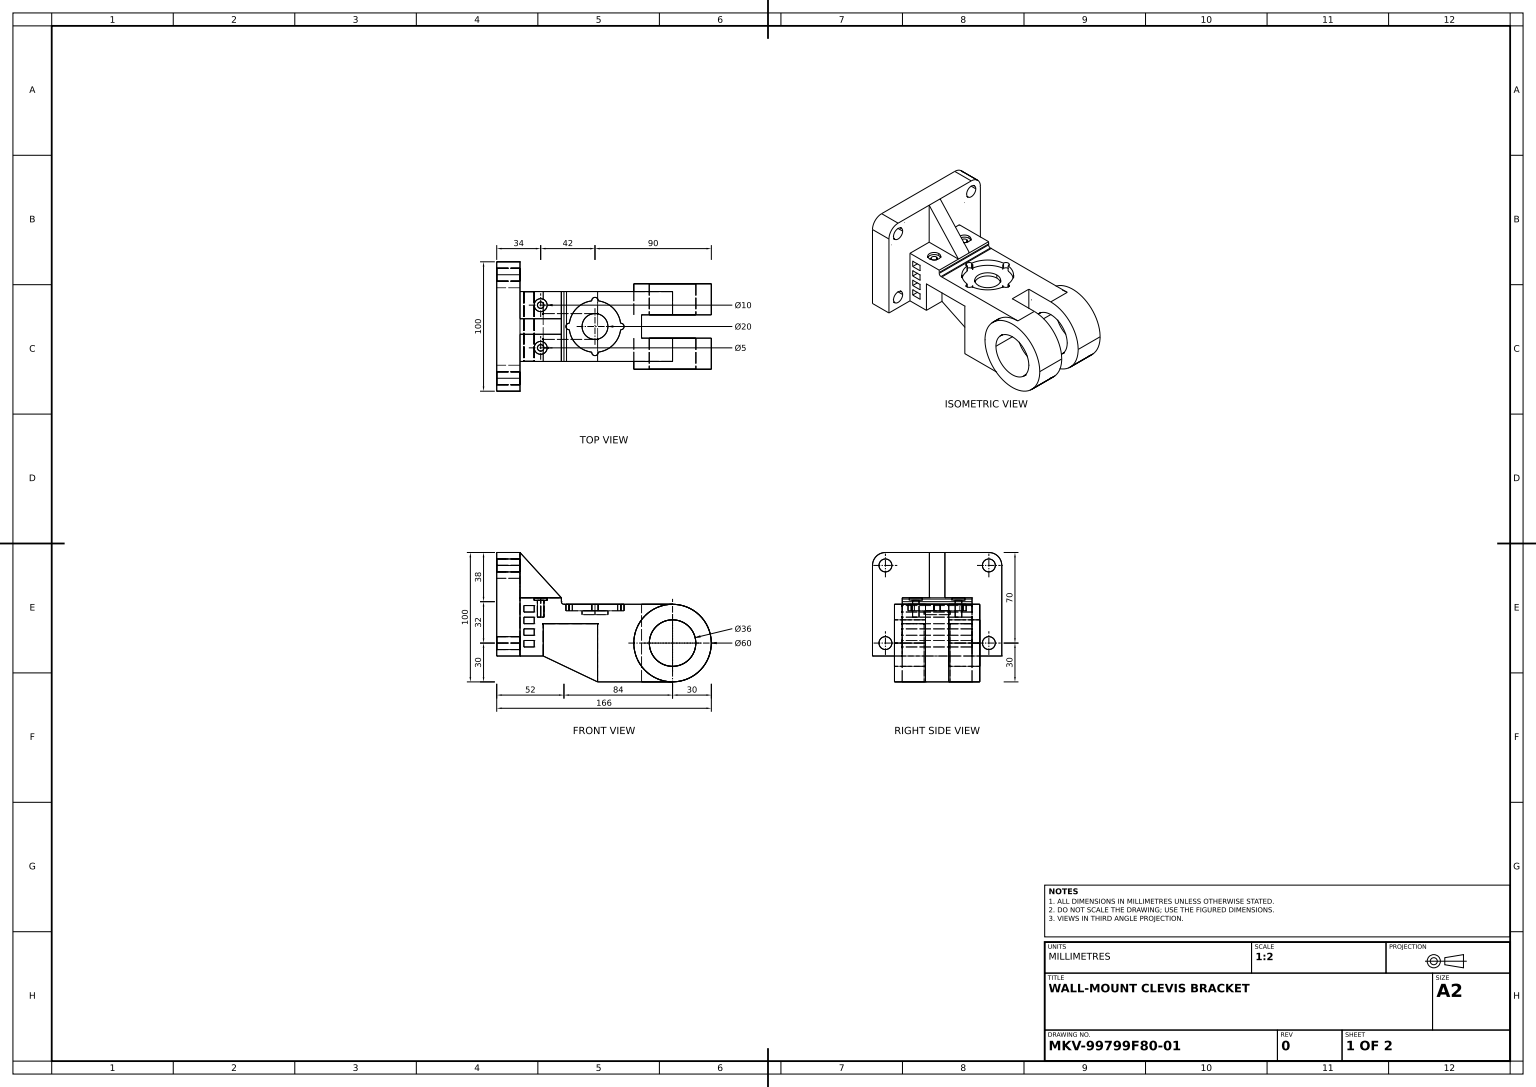
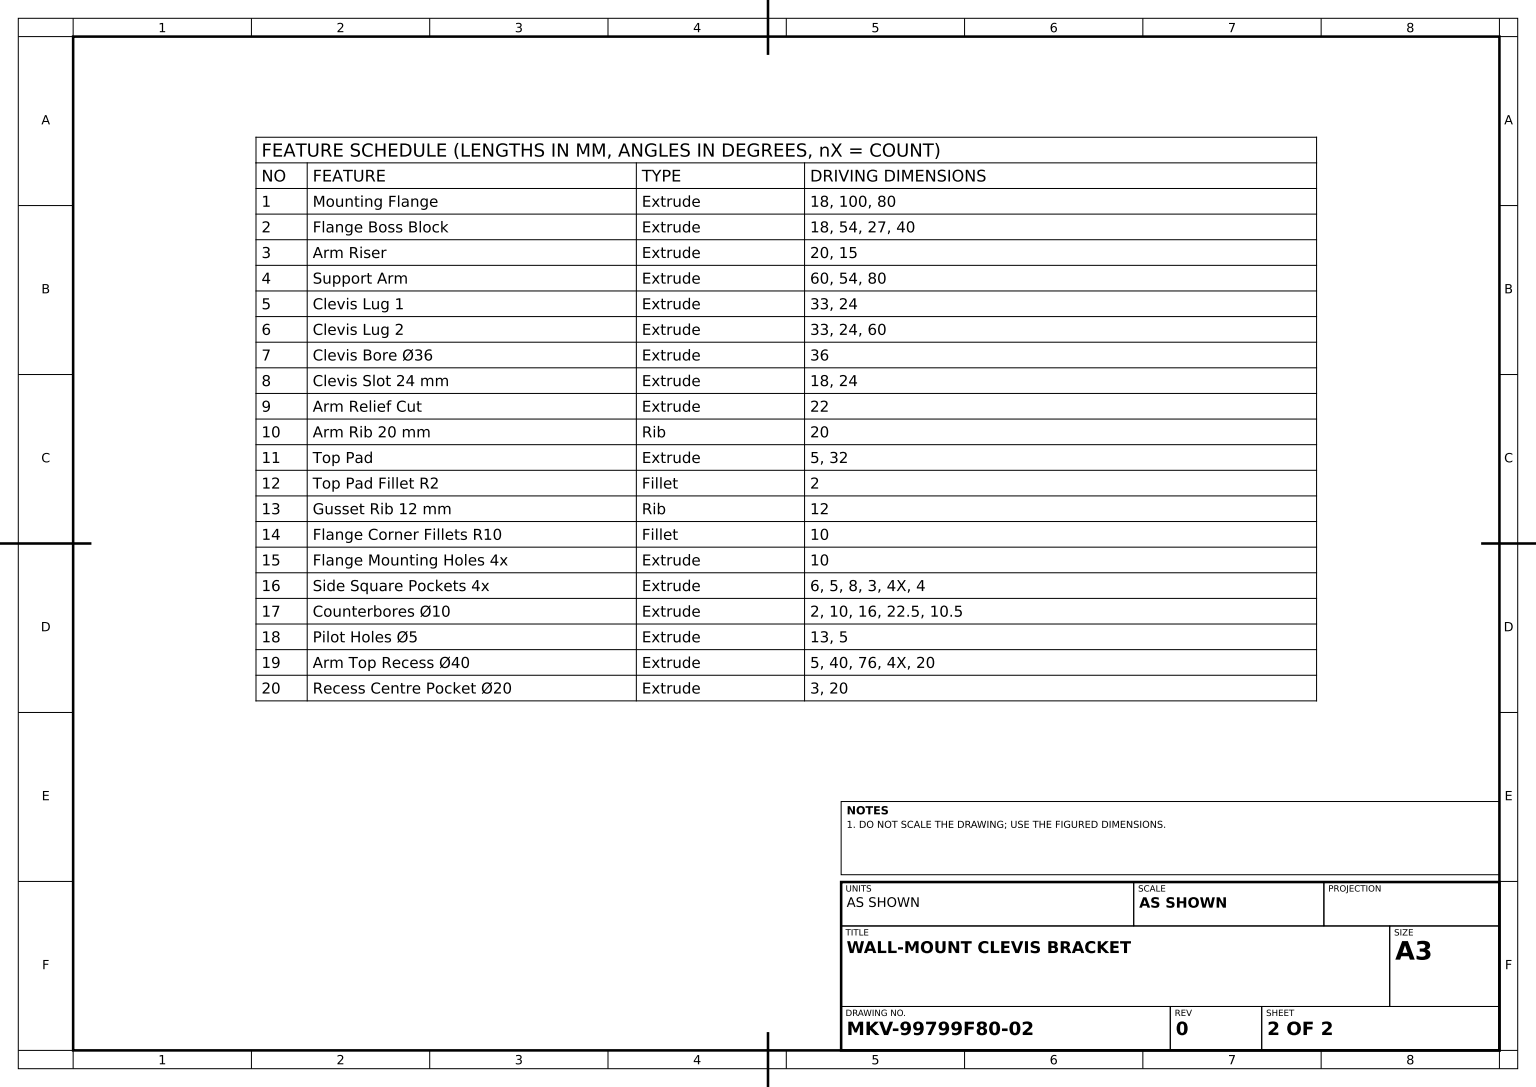
from build123d import *

# Parameters (mm, degrees)
MOUNTING_FLANGE_SKETCH_W          = 100
MOUNTING_FLANGE_SKETCH_H          = 80
MOUNTING_FLANGE_DEPTH             = 18
FLANGE_BOSS_BLOCK_SKETCH_W        = 54
FLANGE_BOSS_BLOCK_SKETCH_H        = 40
FLANGE_BOSS_BLOCK_DEPTH           = 18
ARM_RISER_SKETCH_W                = 54
ARM_RISER_SKETCH_H                = 15
ARM_RISER_DEPTH                   = 20
SUPPORT_ARM_SKETCH_W              = 80
SUPPORT_ARM_SKETCH_H              = 54
SUPPORT_ARM_DEPTH                 = 60
CLEVIS_LUG_1_SKETCH_R             = 30
CLEVIS_LUG_1_DEPTH                = 24
CLEVIS_START                      = 24
CLEVIS_LUG_2_SKETCH_R             = 30
CLEVIS_LUG_2_DEPTH                = 24
CLEVIS_BORE_SKETCH_R              = 18
CLEVIS_BORE_36_DEPTH              = 196.05127531
CLEVIS_SLOT_SKETCH_W              = 24
CLEVIS_SLOT_SKETCH_H              = 18
CLEVIS_SLOT_24_MM_DEPTH           = 184.455716727
ARM_RELIEF_CUT_SKETCH_W           = 22
ARM_RELIEF_CUT_SKETCH_H           = 45
ARM_RELIEF_CUT_DEPTH              = 193.574660846
ARM_RIB_20_MM_REACH               = 185.456
ARM_RIB_SKETCH_WALL_W             = 415.430246854
ARM_RIB_SKETCH_WALL_H             = 20
TOP_PAD_SKETCH_W                  = 32
TOP_PAD_SKETCH_H                  = 54
TOP_PAD_DEPTH                     = 5
TOP_PAD_FILLET_R2_R               = 2
GUSSET_RIB_12_MM_REACH            = 185.456
GUSSET_RIB_SKETCH_WALL_W          = 416.33505626
GUSSET_RIB_SKETCH_WALL_H          = 12
FLANGE_CORNER_FILLETS_R10_R       = 10
FLANGE_MOUNTING_HOLES_SKETCH_R    = 5
FLANGE_MOUNTING_HOLES_4X_DEPTH    = 168.343957166
SIDE_SQUARE_POCKETS_4X_DEPTH      = 193.574660846
SIDE_SQUARE_POCKETS_4X_DEPTH_BACK = 193.574660846
SIDE_SQUARE_POCKETS_SKETCH_W      = 8
SIDE_SQUARE_POCKETS_SKETCH_H      = 5
COUNTERBORE_SKETCH_R              = 5
COUNTERBORES_10_DEPTH             = 2
PILOT_HOLES_SKETCH_R              = 2.5
PILOT_HOLES_5_DEPTH               = 13
ARM_TOP_RECESS_40_DEPTH           = 5
RECESS_CENTRE_POCKET_SKETCH_R     = 10
RECESS_CENTRE_POCKET_20_DEPTH     = 3


with BuildPart() as part:
    # Mounting Flange Sketch → Mounting Flange (new body)
    with BuildSketch(Plane(origin=(0, 0, 0), x_dir=(0, 0, -1), z_dir=(1, 0, 0))):
        Rectangle(MOUNTING_FLANGE_SKETCH_W, MOUNTING_FLANGE_SKETCH_H)
    extrude(amount=MOUNTING_FLANGE_DEPTH)

    # Flange Boss Block Sketch → Flange Boss Block (add)
    with BuildSketch(Plane(origin=(18, 0, 0), x_dir=(0, 0, -1), z_dir=(1, 0, 0))):
        with Locations((0, -20)):
            Rectangle(FLANGE_BOSS_BLOCK_SKETCH_W, FLANGE_BOSS_BLOCK_SKETCH_H)
    extrude(amount=FLANGE_BOSS_BLOCK_DEPTH)

    # Arm Riser Sketch → Arm Riser (add)
    with BuildSketch(Plane(origin=(36, 0, 0), x_dir=(0, 0, -1), z_dir=(1, 0, 0))):
        with Locations((0, -7.5)):
            Rectangle(ARM_RISER_SKETCH_W, ARM_RISER_SKETCH_H)
    extrude(amount=ARM_RISER_DEPTH)

    # Support Arm Sketch → Support Arm (add)
    with BuildSketch(Plane(origin=(0, 0, 0), x_dir=(1, 0, 0), z_dir=(0, 1, 0))):
        with Locations((96, 0)):
            Rectangle(SUPPORT_ARM_SKETCH_W, SUPPORT_ARM_SKETCH_H)
    extrude(amount=-SUPPORT_ARM_DEPTH)

    # Clevis Lug 1 Sketch → Clevis Lug 1 (add)
    with BuildSketch(Plane.XY.offset(33)):
        with Locations((136, -30)):
            Circle(CLEVIS_LUG_1_SKETCH_R)
    extrude(amount=-CLEVIS_LUG_1_DEPTH)

    # Clevis Lug 2 Sketch → Clevis Lug 2 (add)
    with BuildSketch(Plane.XY.offset(-33).offset(CLEVIS_START)):
        with Locations((136, -30)):
            Circle(CLEVIS_LUG_2_SKETCH_R)
    extrude(amount=-CLEVIS_LUG_2_DEPTH)

    # Clevis Bore Sketch → Clevis Bore Ø36 (cut, through all)
    with BuildSketch(Plane.XY.offset(33)):
        with Locations((136, -30)):
            Circle(CLEVIS_BORE_SKETCH_R)
    extrude(amount=-CLEVIS_BORE_36_DEPTH, mode=Mode.SUBTRACT)

    # Clevis Slot Sketch → Clevis Slot 24 mm (cut, through all)
    with BuildSketch(Plane(origin=(0, 0, 0), x_dir=(1, 0, 0), z_dir=(0, 1, 0))):
        with Locations((124, 0)):
            Rectangle(CLEVIS_SLOT_SKETCH_W, CLEVIS_SLOT_SKETCH_H)
    extrude(amount=-CLEVIS_SLOT_24_MM_DEPTH, mode=Mode.SUBTRACT)

    # Arm Relief Cut Sketch → Arm Relief Cut (cut, through all)
    with BuildSketch(Plane.XY.offset(27)):
        with Locations((67, -37.5)):
            Rectangle(ARM_RELIEF_CUT_SKETCH_W, ARM_RELIEF_CUT_SKETCH_H)
    extrude(amount=-ARM_RELIEF_CUT_DEPTH, mode=Mode.SUBTRACT)

    # Arm Rib Sketch wall → Arm Rib 20 mm (add, up to next)
    with BuildSketch(Plane(origin=(57, -50, 0), x_dir=(0.902860518824, -0.429933580392, 0), z_dir=(0.429933580392, 0.902860518824, 0)), mode=Mode.PRIVATE) as arm_rib_20_mm_sk1:
        Rectangle(ARM_RIB_SKETCH_WALL_W, ARM_RIB_SKETCH_WALL_H)
    arm_rib_20_mm_tool1 = extrude(arm_rib_20_mm_sk1.sketch, amount=ARM_RIB_20_MM_REACH, mode=Mode.PRIVATE) - part.part
    add(arm_rib_20_mm_tool1.solids().sort_by_distance((57, -50, 0))[0])

    # Top Pad Sketch → Top Pad (add)
    with BuildSketch(Plane(origin=(0, 0, 0), x_dir=(1, 0, 0), z_dir=(0, 1, 0))):
        with Locations((34, 0)):
            Rectangle(TOP_PAD_SKETCH_W, TOP_PAD_SKETCH_H)
    extrude(amount=TOP_PAD_DEPTH)

    # Top Pad Fillet R2
    top_pad_fillet_r2_edges = [part.edges().sort_by_distance(p)[0] for p in [
        (50, 0, 0),
    ]]
    fillet(top_pad_fillet_r2_edges, radius=TOP_PAD_FILLET_R2_R)

    # Gusset Rib Sketch wall → Gusset Rib 12 mm (add, up to next)
    with BuildSketch(Plane(origin=(34, 22.5, 0), x_dir=(0.674769199545, -0.738028812002, 0), z_dir=(0.738028812002, 0.674769199545, 0)), mode=Mode.PRIVATE) as gusset_rib_12_mm_sk1:
        Rectangle(GUSSET_RIB_SKETCH_WALL_W, GUSSET_RIB_SKETCH_WALL_H)
    gusset_rib_12_mm_tool1 = extrude(gusset_rib_12_mm_sk1.sketch, amount=-GUSSET_RIB_12_MM_REACH, mode=Mode.PRIVATE) - part.part
    add(gusset_rib_12_mm_tool1.solids().sort_by_distance((34, 22.5, 0))[0])

    # Flange Corner Fillets R10
    flange_corner_fillets_r10_edges = [part.edges().sort_by_distance(p)[0] for p in [
        (9, 40, 50),
        (9, 40, -50),
    ]]
    fillet(flange_corner_fillets_r10_edges, radius=FLANGE_CORNER_FILLETS_R10_R)

    # Flange Mounting Holes Sketch → Flange Mounting Holes 4x (cut, through all)
    with BuildSketch(Plane(origin=(18, 0, 0), x_dir=(0, 0, -1), z_dir=(1, 0, 0))):
        with Locations((-40, 30)):
            Circle(FLANGE_MOUNTING_HOLES_SKETCH_R)
        with Locations((40, 30)):
            Circle(FLANGE_MOUNTING_HOLES_SKETCH_R)
        with Locations((-40, -30)):
            Circle(FLANGE_MOUNTING_HOLES_SKETCH_R)
        with Locations((40, -30)):
            Circle(FLANGE_MOUNTING_HOLES_SKETCH_R)
    extrude(amount=-FLANGE_MOUNTING_HOLES_4X_DEPTH, mode=Mode.SUBTRACT)

    # Side Square Pockets Sketch → Side Square Pockets 4x (cut, two sides: drawn at the far end of the back side and taken through both)
    with BuildSketch(Plane.XY.offset(27).offset(-SIDE_SQUARE_POCKETS_4X_DEPTH_BACK)):
        with Locations((25, -3.5)):
            Rectangle(SIDE_SQUARE_POCKETS_SKETCH_W, SIDE_SQUARE_POCKETS_SKETCH_H)
        with Locations((25, -12.5)):
            Rectangle(SIDE_SQUARE_POCKETS_SKETCH_W, SIDE_SQUARE_POCKETS_SKETCH_H)
        with Locations((25, -21.5)):
            Rectangle(SIDE_SQUARE_POCKETS_SKETCH_W, SIDE_SQUARE_POCKETS_SKETCH_H)
        with Locations((25, -30.5)):
            Rectangle(SIDE_SQUARE_POCKETS_SKETCH_W, SIDE_SQUARE_POCKETS_SKETCH_H)
    extrude(amount=SIDE_SQUARE_POCKETS_4X_DEPTH + SIDE_SQUARE_POCKETS_4X_DEPTH_BACK, mode=Mode.SUBTRACT)

    # Counterbore Sketch → Counterbores Ø10 (cut)
    with BuildSketch(Plane(origin=(0, 5, 0), x_dir=(1, 0, 0), z_dir=(0, 1, 0))):
        with Locations(Location((34, -16.5, 0), (0, 0, 270))):
            Circle(COUNTERBORE_SKETCH_R)
        with Locations(Location((34, 16.5, 0), (0, 0, 270))):
            Circle(COUNTERBORE_SKETCH_R)
    extrude(amount=-COUNTERBORES_10_DEPTH, mode=Mode.SUBTRACT)

    # Pilot Holes Sketch → Pilot Holes Ø5 (cut)
    with BuildSketch(Plane(origin=(0, 3, 0), x_dir=(1, 0, 0), z_dir=(0, 1, 0))):
        with Locations(Location((34, 16.5, 0), (0, 0, 270))):
            Circle(PILOT_HOLES_SKETCH_R)
        with Locations(Location((34, -16.5, 0), (0, 0, 270))):
            Circle(PILOT_HOLES_SKETCH_R)
    extrude(amount=-PILOT_HOLES_5_DEPTH, mode=Mode.SUBTRACT)

    # Arm Top Recess Sketch → Arm Top Recess Ø40 (cut)
    with BuildSketch(Plane(origin=(0, 0, 0), x_dir=(1, 0, 0), z_dir=(0, 1, 0))):
        with BuildLine():
            ThreePointArc((73.50488759, 19.84375), (61.857864376, 14.142135624), (56.15625, 2.49511241))
            ThreePointArc((56.15625, 2.49511241), (53.5, 0), (56.15625, -2.49511241))
            ThreePointArc((56.15625, -2.49511241), (61.857864376, -14.142135624), (73.50488759, -19.84375))
            ThreePointArc((73.50488759, -19.84375), (76, -22.5), (78.49511241, -19.84375))
            ThreePointArc((78.49511241, -19.84375), (90.142135624, -14.142135624), (95.84375, -2.49511241))
            ThreePointArc((95.84375, -2.49511241), (98.5, 0), (95.84375, 2.49511241))
            ThreePointArc((95.84375, 2.49511241), (90.142135624, 14.142135624), (78.49511241, 19.84375))
            ThreePointArc((78.49511241, 19.84375), (76, 22.5), (73.50488759, 19.84375))
        make_face()
    extrude(amount=-ARM_TOP_RECESS_40_DEPTH, mode=Mode.SUBTRACT)

    # Recess Centre Pocket Sketch → Recess Centre Pocket Ø20 (cut)
    with BuildSketch(Plane(origin=(0, -5, 0), x_dir=(1, 0, 0), z_dir=(0, 1, 0))):
        with Locations(Location((76, 0, 0), (0, 0, 270))):
            Circle(RECESS_CENTRE_POCKET_SKETCH_R)
    extrude(amount=-RECESS_CENTRE_POCKET_20_DEPTH, mode=Mode.SUBTRACT)


solid = part.part
